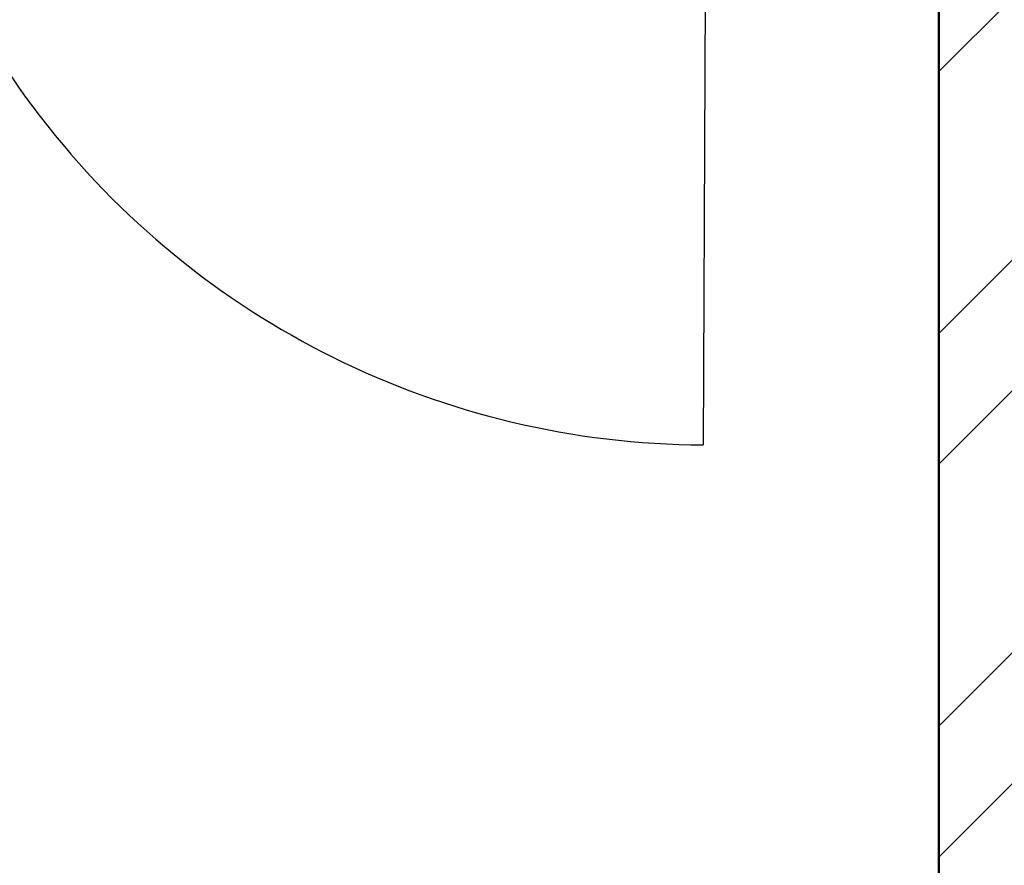
# Model space of a CAD drawing. Units: inches. Extents: x 1901 to 2863, y 888 to 2433.
# Tile 29 of 91: x 2573 to 2607, y 1347 to 1376. Entities that reach past the tile are written whole.
import ezdxf

# ---------------------------------------------------------------- set-up
doc = ezdxf.new("R2010")
doc.units = ezdxf.units.IN
for name, color, linetype, lineweight in [('A-DOOR', 4, 'Continuous', 25), ('A-WALL', 7, 'Continuous', 50), ('A-WALL-PATT', 8, 'Continuous', 13)]:
    doc.layers.add(name, color=color, linetype=linetype, lineweight=lineweight)

# ---------------------------------------------------------------- blocks, each defined once
blk = doc.blocks.new('DOOR-29')
blk.add_line((-0.004, -0.016), (-0.004, 35.984))
blk.add_arc((-0.004, 7.119), 28.865, 345.6888, 90)

msp = doc.modelspace()

# ---------------------------------------------------------------- hatches: boundary and pattern name
at = {"layer": 'A-WALL-PATT'}
h = msp.add_hatch(dxfattribs=at)
h.set_pattern_fill('ANSI32', color=256)
h.paths.add_polyline_path([(2443.926, 2139.888), (2439.426, 2139.888), (2439.426, 2069.348), (2441.676, 2069.348), (2443.926, 2069.348), (2443.926, 2078.634), (2521.926, 2078.634), (2521.926, 2075.067), (2524.176, 2075.067), (2526.426, 2075.067), (2526.426, 2078.634), (2571.755, 2078.634), (2571.755, 2080.884), (2571.755, 2083.134), (2443.926, 2083.134)])
h.paths.add_polyline_path([(2526.426, 2054.634), (2524.176, 2054.634), (2521.926, 2054.634), (2521.926, 2030.634), (2443.926, 2030.634), (2443.926, 2045.348), (2439.426, 2045.348), (2439.426, 1983.867), (2443.926, 1983.867), (2443.926, 2026.134), (2521.926, 2026.134), (2526.426, 2026.134)])
h.paths.add_polyline_path([(2443.926, 1923.867), (2439.426, 1923.867), (2439.426, 1872.634), (2443.926, 1872.634)])
h.paths.add_polyline_path([(2636.233, 1766.134), (2609.926, 1766.134), (2609.926, 1779.785), (2605.426, 1779.785), (2605.426, 1766.134), (2486.614, 1766.134), (2486.614, 1770.671), (2482.114, 1770.671), (2482.114, 1766.134), (2482.114, 1761.634), (2636.233, 1761.634), (2636.233, 1763.884)])
h.paths.add_polyline_path([(2519.536, 1663.384), (2519.536, 1665.634), (2494.926, 1665.634), (2481.831, 1665.634), (2481.831, 1663.384), (2481.831, 1661.134), (2490.426, 1661.134), (2490.426, 1640.157), (2494.926, 1640.157), (2494.926, 1661.134), (2519.536, 1661.134)])
h.paths.add_polyline_path([(2443.926, 1712.134), (2443.926, 1716.634), (2414.464, 1716.634), (2414.464, 1712.134), (2439.426, 1712.134), (2439.426, 1545.507), (2443.926, 1545.507), (2443.926, 1661.134), (2448.475, 1661.134), (2448.475, 1665.634), (2443.926, 1665.634)])
h.paths.add_polyline_path([(2343.426, 1712.134), (2365.525, 1712.134), (2365.525, 1714.384), (2365.525, 1716.634), (2333.871, 1716.634), (2333.871, 1714.384), (2333.871, 1712.134), (2338.926, 1712.134), (2338.926, 1575.634), (2338.926, 1545.507), (2343.426, 1545.507), (2343.426, 1547.507), (2343.426, 1580.134)])
h.paths.add_polyline_path([(2752.926, 1665.634), (2579.536, 1665.634), (2579.536, 1661.134), (2615.926, 1661.134), (2615.926, 1529.134), (2598.931, 1529.134), (2598.931, 1524.634), (2623.127, 1524.634), (2623.127, 1526.884), (2623.127, 1529.134), (2620.426, 1529.134), (2620.426, 1661.134), (2748.426, 1661.134), (2748.426, 1633.499), (2752.926, 1633.499)])
h.paths.add_polyline_path([(2752.926, 1419.929), (2748.426, 1419.929), (2748.426, 1400.134), (2659.426, 1400.134), (2659.426, 1444.333), (2657.176, 1444.333), (2654.926, 1444.333), (2654.926, 1400.134), (2643.649, 1400.134), (2643.649, 1395.634), (2748.426, 1395.634), (2748.426, 1364.035), (2752.926, 1364.035)])
h.paths.add_polyline_path([(2752.926, 1492.878), (2748.426, 1492.878), (2748.426, 1476.634), (2667.426, 1476.634), (2667.426, 1479.71), (2665.176, 1479.71), (2662.926, 1479.71), (2662.926, 1476.634), (2654.926, 1476.634), (2654.926, 1469.536), (2659.426, 1469.536), (2659.426, 1472.134), (2748.426, 1472.134), (2748.426, 1455.929), (2752.926, 1455.929)])
h.paths.add_polyline_path([(2752.926, 1304.035), (2748.426, 1304.035), (2748.426, 1263.634), (2738.66, 1263.634), (2738.66, 1259.134), (2752.926, 1259.134)])
h.paths.add_polyline_path([(2685.926, 1259.134), (2695.49, 1259.134), (2695.49, 1261.384), (2695.49, 1263.634), (2677.837, 1263.634), (2677.837, 1261.384), (2677.837, 1259.134), (2681.426, 1259.134), (2681.426, 1203.634), (2653.277, 1203.634), (2653.277, 1199.134), (2685.926, 1199.134), (2685.926, 1203.634)])
h.paths.add_polyline_path([(2609.426, 1395.634), (2611.848, 1395.634), (2611.848, 1400.134), (2598.888, 1400.134), (2598.888, 1397.884), (2598.888, 1395.634), (2604.926, 1395.634), (2604.926, 1268.134), (2554.726, 1268.134), (2554.726, 1265.884), (2554.726, 1263.634), (2604.926, 1263.634), (2604.926, 1203.634), (2571.306, 1203.634), (2571.306, 1199.134), (2604.926, 1199.134), (2629.277, 1199.134), (2629.277, 1201.384), (2629.277, 1203.634), (2609.426, 1203.634), (2609.426, 1258.634), (2609.426, 1259.134), (2654.804, 1259.134), (2654.804, 1263.634), (2609.426, 1263.634)])
h.paths.add_polyline_path([(2443.926, 1304.035), (2439.426, 1304.035), (2439.426, 1259.134), (2443.926, 1259.134), (2456.16, 1259.134), (2456.16, 1261.384), (2456.16, 1263.634), (2443.926, 1263.634)])
h.paths.add_polyline_path([(2525.426, 1263.634), (2531.778, 1263.634), (2531.778, 1268.134), (2520.926, 1268.134), (2520.926, 1263.634), (2511.409, 1263.634), (2511.409, 1259.134), (2520.926, 1259.134), (2520.926, 1199.134), (2547.306, 1199.134), (2547.306, 1201.384), (2547.306, 1203.634), (2525.426, 1203.634)])
h.paths.add_polyline_path([(2443.926, 1434.842), (2439.426, 1434.842), (2439.426, 1364.035), (2441.676, 1364.035), (2443.926, 1364.035)])
h.paths.add_polyline_path([(2567.134, 1400.134), (2443.926, 1400.134), (2443.926, 1395.634), (2567.134, 1395.634)])
h.paths.add_polyline_path([(2443.926, 1545.507), (2439.426, 1545.507), (2439.426, 1494.842), (2443.926, 1494.842)])
h.paths.add_polyline_path([(2494.926, 1553.349), (2492.676, 1553.349), (2490.426, 1553.349), (2490.426, 1524.634), (2494.926, 1524.634), (2525.936, 1524.634), (2525.936, 1526.884), (2525.936, 1529.134), (2494.926, 1529.134)])
h.paths.add_polyline_path([(2752.926, 1573.499), (2748.426, 1573.499), (2748.426, 1529.134), (2657.759, 1529.134), (2657.759, 1524.634), (2662.926, 1524.634), (2662.926, 1498.631), (2667.426, 1498.631), (2667.426, 1524.634), (2748.426, 1524.634), (2748.426, 1516.878), (2752.926, 1516.878)])
h.paths.add_polyline_path([(2038.602, 2237.418), (2080.174, 2237.418), (2080.174, 2256.075), (2038.602, 2256.075)], flags=9)
h.paths.add_polyline_path([(2292.009, 1062.394), (2539.932, 1062.394), (2539.932, 1099.487), (2292.009, 1099.487)], flags=9)
h.paths.add_polyline_path([(2424.91, 1832.253), (2448.513, 1832.253), (2448.513, 1846.678), (2424.91, 1846.678)], flags=9)
h.paths.add_polyline_path([(2359.076, 1832.253), (2382.678, 1832.253), (2382.678, 1846.678), (2359.076, 1846.678)], flags=9)
h.paths.add_polyline_path([(2352.899, 1684.802), (2367.543, 1684.802), (2367.543, 1697.167), (2352.899, 1697.167)], flags=9)
h.paths.add_polyline_path([(2079.288, 1755.826), (2169.024, 1755.826), (2169.024, 1774.372), (2079.288, 1774.372)], flags=9)
h.paths.add_polyline_path([(2404.09, 1373.857), (2404.09, 1463.593), (2385.544, 1463.593), (2385.544, 1373.857)], flags=9)
h.paths.add_polyline_path([(2268.091, 2236.371), (2309.636, 2236.371), (2309.636, 2255.028), (2268.091, 2255.028)], flags=9)
h.paths.add_polyline_path([(2575.96, 1700.951), (2665.696, 1700.951), (2665.696, 1719.498), (2575.96, 1719.498)], flags=9)
h.paths.add_polyline_path([(2302.962, 1878.474), (2329.524, 1878.474), (2329.524, 1888.777), (2302.962, 1888.777)], flags=9)
h.paths.add_polyline_path([(2097.415, 2240.576), (2126.573, 2240.576), (2126.573, 2259.233), (2097.415, 2259.233)], flags=9)
h.paths.add_polyline_path([(2208.725, 2246.124), (2237.882, 2246.124), (2237.882, 2264.781), (2208.725, 2264.781)], flags=9)
h.paths.add_polyline_path([(2038.147, 1925.958), (2076.987, 1925.958), (2076.987, 1944.615), (2038.147, 1944.615)], flags=9)
h.paths.add_polyline_path([(2239.144, 1926.672), (2288.465, 1926.672), (2288.465, 1945.329), (2239.144, 1945.329)], flags=9)
h.paths.add_polyline_path([(2175.429, 2007.33), (2212.356, 2007.33), (2212.356, 2025.987), (2175.429, 2025.987)], flags=9)
h.paths.add_polyline_path([(2225.034, 2091.794), (2263.875, 2091.794), (2263.875, 2110.451), (2225.034, 2110.451)], flags=9)
h.paths.add_polyline_path([(2035.398, 2098.478), (2074.238, 2098.478), (2074.238, 2117.135), (2035.398, 2117.135)], flags=9)
h.paths.add_polyline_path([(2050.102, 2029.209), (2083.26, 2029.209), (2083.26, 2047.866), (2050.102, 2047.866)], flags=9)
h.paths.add_polyline_path([(2069.677, 1956.719), (2098.835, 1956.719), (2098.835, 1975.376), (2069.677, 1975.376)], flags=9)
h.paths.add_polyline_path([(2328.62, 1753.336), (2361.663, 1753.336), (2361.663, 1771.993), (2328.62, 1771.993)], flags=9)
h.paths.add_polyline_path([(2395.162, 2060.888), (2395.162, 2140.654), (2378.676, 2140.654), (2378.676, 2060.888)], flags=9)
h.paths.add_polyline_path([(2463.728, 2059.02), (2492.886, 2059.02), (2492.886, 2077.677), (2463.728, 2077.677)], flags=9)
h.paths.add_polyline_path([(2458.027, 2181.536), (2496.868, 2181.536), (2496.868, 2200.194), (2458.027, 2200.194)], flags=9)
h.paths.add_polyline_path([(2456.855, 2228.831), (2498.401, 2228.831), (2498.401, 2247.488), (2456.855, 2247.488)], flags=9)
h.paths.add_polyline_path([(2527.577, 2243.074), (2556.735, 2243.074), (2556.735, 2261.731), (2527.577, 2261.731)], flags=9)
h.paths.add_polyline_path([(2694.461, 2232.767), (2736.033, 2232.767), (2736.033, 2251.425), (2694.461, 2251.425)], flags=9)
h.paths.add_polyline_path([(2637.821, 2249.225), (2666.979, 2249.225), (2666.979, 2267.882), (2637.821, 2267.882)], flags=9)
h.paths.add_polyline_path([(2623.687, 2183.541), (2662.528, 2183.541), (2662.528, 2202.199), (2623.687, 2202.199)], flags=9)
h.paths.add_polyline_path([(2691.965, 2021.5), (2725.124, 2021.5), (2725.124, 2040.157), (2691.965, 2040.157)], flags=9)
h.paths.add_polyline_path([(2621.043, 1975.912), (2662.335, 1975.912), (2662.335, 1994.569), (2621.043, 1994.569)], flags=9)
h.paths.add_polyline_path([(2479.032, 1927.62), (2519.844, 1927.62), (2519.844, 1946.277), (2479.032, 1946.277)], flags=9)
h.paths.add_polyline_path([(2670.941, 1849.076), (2716.005, 1849.076), (2716.005, 1867.734), (2670.941, 1867.734)], flags=9)
h.paths.add_polyline_path([(2523.613, 1782.956), (2550.175, 1782.956), (2550.175, 1793.26), (2523.613, 1793.26)], flags=9)
h.paths.add_polyline_path([(2450.841, 1207.331), (2492.386, 1207.331), (2492.386, 1225.989), (2450.841, 1225.989)], flags=9)
h.paths.add_polyline_path([(2527.751, 1203.841), (2556.908, 1203.841), (2556.908, 1222.499), (2527.751, 1222.499)], flags=9)
h.paths.add_polyline_path([(2639.111, 1207.2), (2668.268, 1207.2), (2668.268, 1225.857), (2639.111, 1225.857)], flags=9)
h.paths.add_polyline_path([(2692.594, 1218.965), (2734.167, 1218.965), (2734.167, 1237.623), (2692.594, 1237.623)], flags=9)
h.paths.add_polyline_path([(2669.266, 1366.329), (2708.106, 1366.329), (2708.106, 1384.987), (2669.266, 1384.987)], flags=25)
h.paths.add_polyline_path([(2463.313, 1358.031), (2502.153, 1358.031), (2502.153, 1376.688), (2463.313, 1376.688)], flags=9)
h.paths.add_polyline_path([(2494.725, 1449.963), (2531.652, 1449.963), (2531.652, 1468.62), (2494.725, 1468.62)], flags=9)
h.paths.add_polyline_path([(2675.565, 1422.157), (2708.724, 1422.157), (2708.724, 1440.815), (2675.565, 1440.815)], flags=25)
h.paths.add_polyline_path([(2685.634, 1493.891), (2714.792, 1493.891), (2714.792, 1512.548), (2685.634, 1512.548)], flags=9)
h.paths.add_polyline_path([(2686.805, 1529.913), (2725.645, 1529.913), (2725.645, 1548.57), (2686.805, 1548.57)], flags=25)
h.paths.add_polyline_path([(2503.651, 1537.991), (2552.972, 1537.991), (2552.972, 1556.648), (2503.651, 1556.648)], flags=9)
h.paths.add_polyline_path([(2291.713, 1643.504), (2318.275, 1643.504), (2318.275, 1653.807), (2291.713, 1653.807)], flags=9)
h.paths.add_polyline_path([(2450.626, 1610.52), (2477.189, 1610.52), (2477.189, 1620.824), (2450.626, 1620.824)], flags=9)
h.paths.add_polyline_path([(2359.985, 1551.814), (2422.253, 1551.814), (2422.253, 1562.117), (2359.985, 1562.117)], flags=9)
h.paths.add_polyline_path([(2280.106, 1249.006), (2321.651, 1249.006), (2321.651, 1267.663), (2280.106, 1267.663)], flags=9)
h.paths.add_polyline_path([(2164.057, 1274.232), (2193.215, 1274.232), (2193.215, 1292.889), (2164.057, 1292.889)], flags=9)
h.paths.add_polyline_path([(2118.21, 1277.694), (2151.252, 1277.694), (2151.252, 1296.351), (2118.21, 1296.351)], flags=9)
h.paths.add_polyline_path([(2031.946, 1268.529), (2073.519, 1268.529), (2073.519, 1287.187), (2031.946, 1287.187)], flags=9)
h.paths.add_polyline_path([(2050.199, 1409.079), (2089.04, 1409.079), (2089.04, 1427.736), (2050.199, 1427.736)], flags=9)
h.paths.add_polyline_path([(2243.743, 1421.032), (2282.584, 1421.032), (2282.584, 1439.689), (2243.743, 1439.689)], flags=9)
h.paths.add_polyline_path([(2190.746, 1509.769), (2231.558, 1509.769), (2231.558, 1528.426), (2190.746, 1528.426)], flags=9)
h.paths.add_polyline_path([(2058.392, 1475.415), (2091.55, 1475.415), (2091.55, 1494.073), (2058.392, 1494.073)], flags=9)
h.paths.add_polyline_path([(2062.447, 1553.09), (2091.605, 1553.09), (2091.605, 1571.747), (2062.447, 1571.747)], flags=9)
h.paths.add_polyline_path([(2219.524, 1590.365), (2266.147, 1590.365), (2266.147, 1609.022), (2219.524, 1609.022)], flags=9)
h.paths.add_polyline_path([(2041.072, 1584.188), (2079.912, 1584.188), (2079.912, 1602.845), (2041.072, 1602.845)], flags=9)

# ---------------------------------------------------------------- linework, layer by layer
at = {"layer": 'A-WALL'}
msp.add_line((2604.926, 1395.634), (2604.926, 1268.134), dxfattribs=at)

# ---------------------------------------------------------------- block references
at = {"layer": 'A-DOOR', "rotation": 179.7338121645225}
msp.add_blockref('DOOR-29', (2597.001, 1397.808), dxfattribs=at)

doc.saveas('drawing.dxf')
